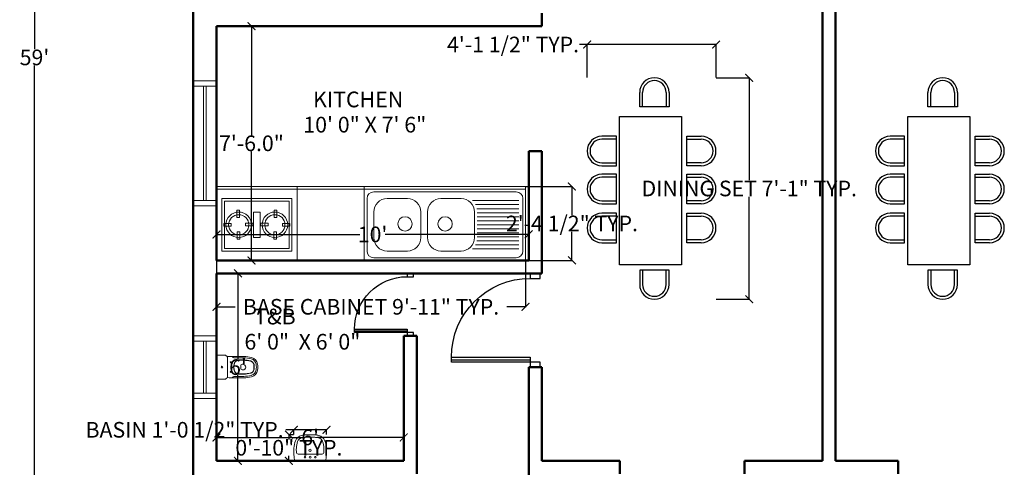
# Model space of a CAD drawing. Units: inches. Extents: x 147 to 1638, y 107 to 941.
# Tile 8 of 17: x 158 to 537, y 398 to 570. Entities that reach past the tile are written whole.
import ezdxf

# ---------------------------------------------------------------- set-up
doc = ezdxf.new("R2010")
doc.units = ezdxf.units.IN
doc.header["$MEASUREMENT"] = 0
for name, color, linetype, lineweight in [('A-ANNO-DIMS', 2, 'Continuous', 15), ('A-AREA-IDEN', 7, 'Continuous', 18), ('A-Door', 150, 'Continuous', 25), ('A-EQPM', 8, 'Continuous', 18), ('A-FLOR-CASE', 9, 'Continuous', 20), ('A-FLOR-FIXT', 9, 'Continuous', 18), ('furniture', 50, 'Continuous', 18), ('walls', 7, 'Continuous', 50), ('windows', 3, 'Continuous', 20)]:
    doc.layers.add(name, color=color, linetype=linetype, lineweight=lineweight)
for name, color, linetype in [('A-Glaz', 92, 'Continuous'), ('NT', 1, 'Continuous'), ('家', 40, 'Continuous')]:
    doc.layers.add(name, color=color, linetype=linetype)
doc.styles.get("Standard").update_dxf_attribs({"font": 'arial.ttf'})
doc.dimstyles.get("Standard").update_dxf_attribs({"dimtxt": 6, "dimasz": 3, "dimexe": 0.18, "dimexo": 0.0625, "dimgap": 0.09, "dimtad": 0, "dimtih": 1, "dimtoh": 1, "dimdec": 1, "dimzin": 0, "dimdsep": 46, "dimlunit": 3, "dimtxsty": 'Standard', "dimblk": 'ARCHTICK', "dimcen": 0.09, "dimadec": 0, "dimazin": 0, "dimtfac": 1, "dimtdec": 1, "dimtofl": 0, "dimtmove": 0, "dimatfit": 3, "dimfxl": 1, "dimtolj": 1, "dimtzin": 0, "dimarcsym": 0})

# ---------------------------------------------------------------- blocks, each defined once
blk = doc.blocks.new('A$C087A3AA9')
at = {"layer": 'A-Door'}
for points in [[(852.6, 94.7), (852.6, 852.6), (805.3, 852.6), (805.3, 94.7)], [(47.4, 94.7), (47.4, 0), (0, 0), (0, 94.7)], [(900, 94.7), (900, 0), (852.6, 0), (852.6, 94.7)]]:
    blk.add_lwpolyline(points, close=True, dxfattribs=at)
at = {"layer": 'A-Glaz'}
blk.add_line((828.9, 852.6), (828.9, 94.7), dxfattribs=at)
at = {"layer": 'NT'}
blk.add_arc((805.3, 94.7), 757.9, 90, 180, dxfattribs=at)
blk = doc.blocks.new('_ArchTick')
at = {"color": 0, "linetype": 'ByBlock', "const_width": 0.15}
blk.add_lwpolyline([(-0.5, -0.5), (0.5, 0.5)], dxfattribs=at)
blk = doc.blocks.new('*D14')
at = {"layer": 'A-ANNO-DIMS', "color": 0, "lineweight": -2, "transparency": 16777216}
for p, q in [((244.71, 567.72), (247.56, 567.72)), ((247.38, 567.72), (247.38, 525.87)), ((247.38, 477.72), (247.38, 519.56)), ((244.71, 477.72), (247.56, 477.72))]:
    blk.add_line(p, q, dxfattribs=at)
at = {"layer": 'Defpoints', "color": 0, "lineweight": -2, "transparency": 16777216}
for p in [(244.65, 567.72), (244.65, 477.72), (247.38, 477.72)]:
    blk.add_point(p, dxfattribs=at)
at = {"layer": 'A-ANNO-DIMS', "color": 0, "lineweight": -2, "transparency": 16777216, "xscale": 3, "yscale": 3, "zscale": 3}
for p, rotation in [((247.38, 567.72), 90), ((247.38, 477.72), 270)]:
    blk.add_blockref('_ArchTick', p, dxfattribs=dict(at, rotation=rotation))
at = {"layer": 'A-ANNO-DIMS', "color": 0, "transparency": 16777216, "insert": (247.38, 522.72), "char_height": 6, "attachment_point": 5}
blk.add_mtext('\\A1;7\'-6.0"', dxfattribs=at)
blk = doc.blocks.new('*D15')
at = {"layer": 'A-ANNO-DIMS', "color": 0, "lineweight": -2, "transparency": 16777216}
for p, q in [((233.94, 487.78), (233.94, 487.9)), ((233.94, 487.72), (289.05, 487.72)), ((353.94, 487.72), (298.84, 487.72)), ((353.94, 487.78), (353.94, 487.9))]:
    blk.add_line(p, q, dxfattribs=at)
at = {"layer": 'Defpoints', "color": 0, "lineweight": -2, "transparency": 16777216}
for p in [(233.94, 487.72), (353.94, 487.72), (353.94, 487.72)]:
    blk.add_point(p, dxfattribs=at)
at = {"layer": 'A-ANNO-DIMS', "color": 0, "lineweight": -2, "transparency": 16777216, "xscale": 3, "yscale": 3, "zscale": 3, "rotation": 180}
blk.add_blockref('_ArchTick', (233.94, 487.72), dxfattribs=at)
at = {"layer": 'A-ANNO-DIMS', "color": 0, "lineweight": -2, "transparency": 16777216, "xscale": 3, "yscale": 3, "zscale": 3}
blk.add_blockref('_ArchTick', (353.94, 487.72), dxfattribs=at)
at = {"layer": 'A-ANNO-DIMS', "color": 0, "transparency": 16777216, "insert": (293.94, 487.72), "char_height": 6, "attachment_point": 5}
blk.add_mtext("\\A1;10'", dxfattribs=at)
blk = doc.blocks.new('*D16')
at = {"layer": 'A-ANNO-DIMS', "color": 0, "lineweight": -2, "transparency": 16777216}
for p, q in [((239.65, 472.72), (242.37, 472.72)), ((242.19, 472.72), (242.19, 439.87)), ((242.19, 400.72), (242.19, 433.56)), ((239.65, 400.72), (242.37, 400.72))]:
    blk.add_line(p, q, dxfattribs=at)
at = {"layer": 'Defpoints', "color": 0, "lineweight": -2, "transparency": 16777216}
for p in [(239.59, 472.72), (239.59, 400.72), (242.19, 400.72)]:
    blk.add_point(p, dxfattribs=at)
at = {"layer": 'A-ANNO-DIMS', "color": 0, "lineweight": -2, "transparency": 16777216, "xscale": 3, "yscale": 3, "zscale": 3}
for p, rotation in [((242.19, 472.72), 90), ((242.19, 400.72), 270)]:
    blk.add_blockref('_ArchTick', p, dxfattribs=dict(at, rotation=rotation))
at = {"layer": 'A-ANNO-DIMS', "color": 0, "transparency": 16777216, "insert": (242.19, 436.72), "char_height": 6, "attachment_point": 5}
blk.add_mtext("\\A1;6'", dxfattribs=at)
blk = doc.blocks.new('*D17')
at = {"layer": 'A-ANNO-DIMS', "color": 0, "lineweight": -2, "transparency": 16777216}
for p, q in [((233.94, 407.58), (233.94, 409.9)), ((233.94, 409.72), (267.08, 409.72)), ((305.94, 409.72), (272.81, 409.72)), ((305.94, 407.58), (305.94, 409.9))]:
    blk.add_line(p, q, dxfattribs=at)
at = {"layer": 'Defpoints', "color": 0, "lineweight": -2, "transparency": 16777216}
for p in [(305.94, 409.72), (233.94, 407.52), (305.94, 407.52)]:
    blk.add_point(p, dxfattribs=at)
at = {"layer": 'A-ANNO-DIMS', "color": 0, "lineweight": -2, "transparency": 16777216, "xscale": 3, "yscale": 3, "zscale": 3, "rotation": 180}
blk.add_blockref('_ArchTick', (233.94, 409.72), dxfattribs=at)
at = {"layer": 'A-ANNO-DIMS', "color": 0, "lineweight": -2, "transparency": 16777216, "xscale": 3, "yscale": 3, "zscale": 3}
blk.add_blockref('_ArchTick', (305.94, 409.72), dxfattribs=at)
at = {"layer": 'A-ANNO-DIMS', "color": 0, "transparency": 16777216, "insert": (269.94, 409.72), "char_height": 6, "attachment_point": 5}
blk.add_mtext("\\A1;6'", dxfattribs=at)
blk = doc.blocks.new('*D70')
at = {"layer": 'A-ANNO-DIMS', "color": 0, "lineweight": -2, "transparency": 16777216}
for p, q in [((224.88, 909.72), (163.8, 909.72)), ((163.98, 909.72), (163.98, 558.87)), ((163.98, 201.72), (163.98, 552.56)), ((224.88, 201.72), (163.8, 201.72))]:
    blk.add_line(p, q, dxfattribs=at)
at = {"layer": 'Defpoints', "color": 0, "lineweight": -2, "transparency": 16777216}
for p in [(224.94, 909.72), (163.98, 201.72), (224.94, 201.72)]:
    blk.add_point(p, dxfattribs=at)
at = {"layer": 'A-ANNO-DIMS', "color": 0, "lineweight": -2, "transparency": 16777216, "xscale": 3, "yscale": 3, "zscale": 3}
for p, rotation in [((163.98, 909.72), 90), ((163.98, 201.72), 270)]:
    blk.add_blockref('_ArchTick', p, dxfattribs=dict(at, rotation=rotation))
at = {"layer": 'A-ANNO-DIMS', "color": 0, "transparency": 16777216, "insert": (163.98, 555.72), "char_height": 6, "attachment_point": 5}
blk.add_mtext("\\A1;59'", dxfattribs=at)
blk = doc.blocks.new('2SAINDA')
at = {"color": 0, "linetype": 'ByBlock'}
for p, q in [((0, 0.188), (0, -0.188)), ((0.018, 0.2), (0.141, 0.2)), ((0.157, 0.192), (0.162, 0.188)), ((0.18, -0.164), (0.18, 0.164)), ((0.279, 0.159), (0.261, 0.176)), ((0.437, 0.047), (0.424, 0.047)), ((0.279, -0.159), (0.261, -0.176)), ((0.437, -0.047), (0.424, -0.047)), ((0.018, -0.2), (0.141, -0.2)), ((0.157, -0.192), (0.162, -0.188))]:
    blk.add_line(p, q, dxfattribs=at)
for centre, radius in [((0.09, 0), 0.0135), ((0.09, 0), 0.0135), ((0.236, 0.08), 0.0075), ((0.236, -0.08), 0.0075)]:
    blk.add_circle(centre, radius, dxfattribs=at)
for centre, radius, start, end in [((0.018, 0.18), 0.02, 90, 155.6901), ((0.141, 0.181), 0.019, 34.9372, 90), ((0.155, 0.164), 0.025, 23.3776, 73.7848), ((0.383, -5.322), 5.5, 89.2905, 92.1362), ((0.155, 0.164), 0.025, 360, 23.3776), ((0.444, -0.373), 0.55, 75.4605, 89.2905), ((0.293, 0.173), 0.02, 225, 270.9364), ((0.485, 0), 0.2, 160.016, 199.984), ((0.485, 0), 0.196, 160.016, 199.984), ((0.383, -5.322), 5.476, 89.2905, 90.9364), ((0.368, 0.043), 0.075, 90.1648, 160.016), ((0.368, 0.043), 0.071, 90.1648, 160.016), ((0.383, -5.322), 5.44, 89.2905, 90.1648), ((0.383, -5.322), 5.436, 89.2905, 90.1648), ((0.582, 0), 0.18, 170.2849, 189.7151), ((0.424, 0.027), 0.02, 90, 170.2849), ((0.437, 0), 0.047, 0, 90), ((0.437, 0), 0.047, 270, 0), ((0.444, -0.373), 0.49, 75.4605, 89.2905), ((0.444, -0.373), 0.486, 75.4605, 89.2905), ((0.444, -0.373), 0.526, 75.4605, 89.2905), ((0.549, 0.03), 0.07, 8.8162, 75.4605), ((0.549, 0.03), 0.074, 8.8162, 75.4605), ((0.549, 0.03), 0.11, 8.8162, 75.4605), ((0.549, 0.03), 0.134, 8.8162, 75.4605), ((0.355, 0), 0.266, 351.1838, 8.8162), ((0.355, 0), 0.27, 351.1838, 8.8162), ((0.355, 0), 0.306, 351.1838, 8.8162), ((0.355, 0), 0.33, 351.1838, 8.8162), ((0.293, -0.173), 0.02, 89.0636, 135), ((0.383, 5.322), 5.476, 269.0636, 270.7095), ((0.368, -0.043), 0.075, 199.984, 269.8352), ((0.368, -0.043), 0.071, 199.984, 269.8352), ((0.383, 5.322), 5.436, 269.8352, 270.7095), ((0.383, 5.322), 5.44, 269.8352, 270.7095), ((0.424, -0.027), 0.02, 189.7151, 270), ((0.444, 0.373), 0.486, 270.7095, 284.5395), ((0.444, 0.373), 0.49, 270.7095, 284.5395), ((0.444, 0.373), 0.526, 270.7095, 284.5395), ((0.444, 0.373), 0.55, 270.7095, 284.5395), ((0.549, -0.03), 0.07, 284.5395, 351.1838), ((0.549, -0.03), 0.074, 284.5395, 351.1838), ((0.549, -0.03), 0.11, 284.5395, 351.1838), ((0.549, -0.03), 0.134, 284.5395, 351.1838), ((0.018, -0.18), 0.02, 204.3099, 270), ((0.141, -0.181), 0.019, 270, 325.0628), ((0.155, -0.164), 0.025, 286.2152, 336.6224), ((0.155, -0.164), 0.025, 336.6224, 0), ((0.383, 5.322), 5.5, 267.8638, 270.7095)]:
    blk.add_arc(centre, radius, start, end, dxfattribs=at)
blk = doc.blocks.new('2SALADA2')
at = {"color": 0}
for p, q in [((-0.296, 0), (0.296, 0)), ((0.207, -0.13), (-0.207, -0.13))]:
    blk.add_line(p, q, dxfattribs=at)
for centre, radius in [((-0.1, -0.07), 0.015), ((0, -0.205), 0.023), ((0, -0.07), 0.0175), ((0.1, -0.07), 0.015)]:
    blk.add_circle(centre, radius, dxfattribs=at)
for centre, radius, start, end in [((-0.296, -0.01), 0.01, 90, 173.6262), ((0.296, -0.01), 0.01, 6.3738, 90), ((1.185, -0.175), 1.5, 173.6262, 182.693), ((1.186, -0.221), 1.454, 178.0234, 180.898), ((-0.227, -0.171), 0.04, 95.5937, 179.6995), ((-0.207, -0.38), 0.25, 90, 95.5937), ((0.207, -0.38), 0.25, 84.4063, 90), ((0.227, -0.171), 0.04, 0.3005, 84.4063), ((-1.186, -0.221), 1.454, 359.102, 1.9766), ((-1.185, -0.175), 1.5, 357.307, 6.3738), ((0.186, -0.222), 0.5, 182.693, 199.3406), ((0.186, -0.222), 0.454, 182.693, 199.3406), ((-0.135, -0.335), 0.114, 199.3406, 257.4429), ((0.135, -0.335), 0.114, 282.5571, 340.6594), ((-0.186, -0.222), 0.454, 340.6594, 357.307), ((-0.186, -0.222), 0.5, 340.6594, 357.307), ((-0.135, -0.335), 0.16, 199.3406, 257.4429), ((-0.061, -0.003), 0.5, 257.4429, 266.4982), ((-0.061, -0.003), 0.454, 257.4429, 266.4982), ((0, 0.995), 1.5, 266.4982, 273.5018), ((0, 0.995), 1.454, 266.4982, 273.5018), ((0.061, -0.003), 0.454, 273.5018, 282.5571), ((0.061, -0.003), 0.5, 273.5018, 282.5571), ((0.135, -0.335), 0.16, 282.5571, 340.6594)]:
    blk.add_arc(centre, radius, start, end, dxfattribs=at)
blk = doc.blocks.new('A$C45A766E2')
at = {"layer": '家'}
for p, q in [((0.363, 1.317), (0.363, 1.078)), ((0.412, 1.317), (0.412, 1.078)), ((0.801, 1.078), (0.801, 1.317)), ((0.849, 1.078), (0.849, 1.317)), ((1.006, 1.317), (1.006, 1.078)), ((1.054, 1.317), (1.054, 1.078)), ((1.443, 1.078), (1.443, 1.317)), ((1.492, 1.078), (1.492, 1.317)), ((1.634, 1.317), (1.634, 1.078)), ((1.683, 1.317), (1.683, 1.078)), ((2.072, 1.078), (2.072, 1.317)), ((2.12, 1.078), (2.12, 1.317)), ((0, 1.028), (2.445, 1.028)), ((0, 0), (0, 1.028)), ((0.363, 1.078), (0.849, 1.078)), ((0.363, 1.078), (0.849, 1.078)), ((1.006, 1.078), (1.492, 1.078)), ((1.006, 1.078), (1.492, 1.078)), ((1.634, 1.078), (2.12, 1.078)), ((1.634, 1.078), (2.12, 1.078)), ((2.445, 1.028), (2.445, 0)), ((-0.088, 0.693), (-0.327, 0.693)), ((-0.088, 0.207), (-0.088, 0.693)), ((-0.088, 0.207), (-0.088, 0.693)), ((2.604, 0.693), (2.843, 0.693)), ((2.604, 0.207), (2.604, 0.693)), ((2.604, 0.207), (2.604, 0.693)), ((-0.088, 0.644), (-0.327, 0.644)), ((2.604, 0.644), (2.843, 0.644)), ((-0.327, 0.255), (-0.088, 0.255)), ((-0.327, 0.207), (-0.088, 0.207)), ((2.843, 0.255), (2.604, 0.255)), ((2.843, 0.207), (2.604, 0.207)), ((2.445, 0), (0, 0)), ((0.363, -0.085), (0.849, -0.085)), ((0.363, -0.085), (0.849, -0.085)), ((0.363, -0.324), (0.363, -0.085)), ((0.412, -0.324), (0.412, -0.085)), ((0.801, -0.085), (0.801, -0.324)), ((0.849, -0.085), (0.849, -0.324)), ((1.006, -0.324), (1.006, -0.085)), ((1.006, -0.085), (1.492, -0.085)), ((1.006, -0.085), (1.492, -0.085)), ((1.054, -0.324), (1.054, -0.085)), ((1.443, -0.085), (1.443, -0.324)), ((1.492, -0.085), (1.492, -0.324)), ((1.634, -0.085), (2.12, -0.085)), ((1.634, -0.085), (2.12, -0.085)), ((1.634, -0.324), (1.634, -0.085)), ((1.683, -0.324), (1.683, -0.085)), ((2.072, -0.085), (2.072, -0.324)), ((2.12, -0.085), (2.12, -0.324))]:
    blk.add_line(p, q, dxfattribs=at)
for centre, radius, start, end in [((0.606, 1.317), 0.243, 0, 180), ((0.606, 1.317), 0.195, 0, 180), ((1.249, 1.317), 0.243, 0, 180), ((1.249, 1.317), 0.195, 0, 180), ((1.877, 1.317), 0.243, 0, 180), ((1.877, 1.317), 0.195, 0, 180), ((-0.327, 0.45), 0.243, 90, 270), ((2.843, 0.45), 0.243, 270, 90), ((-0.327, 0.45), 0.195, 90, 270), ((2.843, 0.45), 0.195, 270, 90), ((0.606, -0.324), 0.243, 180, 0), ((0.606, -0.324), 0.195, 180, 0), ((1.249, -0.324), 0.243, 180, 0), ((1.249, -0.324), 0.195, 180, 0), ((1.877, -0.324), 0.243, 180, 0), ((1.877, -0.324), 0.195, 180, 0)]:
    blk.add_arc(centre, radius, start, end, dxfattribs=at)
blk = doc.blocks.new('WIN-48IN')
for p, q in [((9, 48), (0, 48)), ((0, 48), (0, 0)), ((9, 46), (0, 46)), ((4, 2), (4, 46)), ((5, 2), (5, 46)), ((9, 0), (9, 48)), ((0, 2), (9, 2)), ((0, 0), (9, 0))]:
    blk.add_line(p, q)
blk = doc.blocks.new('WIN-24IN')
for p, q in [((9, 24), (0, 24)), ((0, 24), (0, 0)), ((9, 0), (9, 24)), ((9, 22), (0, 22)), ((4, 2), (4, 22)), ((5, 2), (5, 22)), ((0, 2), (9, 2)), ((0, 0), (9, 0))]:
    blk.add_line(p, q)
blk = doc.blocks.new('CABINET-KITCHEN-RUN')
for p, q in [((0, 28.41), (118.8, 28.41)), ((0, 0), (0, 28.41)), ((0, 27.38), (118.8, 27.38)), ((30.99, 0), (30.99, 28.41)), ((56.82, 0), (56.82, 28.41)), ((118.8, 28.41), (118.8, 0)), ((118.8, 0), (0, 0))]:
    blk.add_line(p, q)
blk = doc.blocks.new('COOKTOP-2-BURNER')
for p, q in [((0, 0), (0, 20.15)), ((0, 20.15), (26.86, 20.15)), ((1.03, 1.03), (1.03, 19.11)), ((1.03, 19.11), (25.83, 19.11)), ((25.83, 1.03), (25.83, 19.11)), ((26.86, 0), (26.86, 20.15)), ((5.75, 15.75), (5.75, 12.91)), ((5.75, 15.75), (6.79, 15.75)), ((6.79, 15.75), (6.79, 12.91)), ((21.11, 15.75), (20.07, 15.75)), ((20.07, 15.75), (20.07, 12.91)), ((21.11, 15.75), (21.11, 12.91)), ((5.75, 12.91), (6.79, 12.91)), ((12.14, 14.98), (14.72, 14.98)), ((12.14, 14.98), (12.14, 5.17)), ((14.72, 14.98), (14.72, 5.17)), ((21.11, 12.91), (20.07, 12.91)), ((0.69, 9.55), (0.69, 10.59)), ((0.69, 10.59), (3.53, 10.59)), ((0.69, 9.55), (3.53, 9.55)), ((3.53, 9.55), (3.53, 10.59)), ((11.95, 10.69), (9.11, 10.69)), ((9.11, 10.69), (9.11, 9.66)), ((11.95, 9.66), (9.11, 9.66)), ((11.95, 10.69), (11.95, 9.66)), ((14.91, 10.69), (17.75, 10.69)), ((14.91, 10.69), (14.91, 9.66)), ((14.91, 9.66), (17.75, 9.66)), ((17.75, 10.69), (17.75, 9.66)), ((23.33, 9.55), (23.33, 10.59)), ((26.17, 10.59), (23.33, 10.59)), ((26.17, 9.55), (23.33, 9.55)), ((26.17, 9.55), (26.17, 10.59)), ((5.86, 4.49), (5.86, 7.33)), ((6.89, 7.33), (5.86, 7.33)), ((6.89, 4.49), (5.86, 4.49)), ((6.89, 4.49), (6.89, 7.33)), ((12.14, 5.17), (14.72, 5.17)), ((19.97, 4.49), (19.97, 7.33)), ((19.97, 7.33), (21, 7.33)), ((19.97, 4.49), (21, 4.49)), ((21, 4.49), (21, 7.33)), ((0, 0), (26.86, 0)), ((1.03, 1.03), (25.83, 1.03))]:
    blk.add_line(p, q)
for centre, radius in [((6.48, 10.08), 4.91), ((6.48, 10.08), 3.87), ((20.38, 10.08), 4.91), ((20.38, 10.08), 3.87)]:
    blk.add_circle(centre, radius)
blk = doc.blocks.new('SINK-DOUBLE-DRAINBOARD')
for p, q in [((0, 22.73), (0, 2.58)), ((57.34, 25.31), (2.58, 25.31)), ((15.5, 22.73), (7.75, 22.73)), ((36.16, 22.73), (28.41, 22.73)), ((59.92, 2.58), (59.92, 22.73)), ((40.53, 21.95), (58.37, 21.95)), ((41.67, 20.4), (58.37, 20.4)), ((2.58, 17.56), (2.58, 7.75)), ((20.66, 17.56), (20.66, 7.75)), ((23.24, 17.56), (23.24, 7.75)), ((41.32, 17.56), (41.32, 7.75)), ((42.22, 18.85), (58.37, 18.85)), ((42.36, 17.3), (58.37, 17.3)), ((42.36, 15.75), (58.37, 15.75)), ((42.36, 14.2), (58.37, 14.2)), ((42.36, 12.66), (58.37, 12.66)), ((42.36, 11.11), (58.37, 11.11)), ((42.36, 9.56), (58.37, 9.56)), ((42.36, 8.01), (58.37, 8.01)), ((41.67, 4.91), (58.37, 4.91)), ((42.22, 6.46), (58.37, 6.46)), ((2.58, 0), (57.34, 0)), ((7.75, 2.58), (15.5, 2.58)), ((28.41, 2.58), (36.16, 2.58)), ((40.53, 3.36), (58.37, 3.36))]:
    blk.add_line(p, q)
for centre in [(14.61, 13), (30.02, 13)]:
    blk.add_circle(centre, 2.75)
for centre, radius, start, end in [((2.58, 22.73), 2.58, 90, 180), ((7.75, 17.56), 5.17, 90, 180), ((15.5, 17.56), 5.17, 0, 90), ((28.41, 17.56), 5.17, 90, 180), ((36.16, 17.56), 5.17, 0, 90), ((57.34, 22.73), 2.58, 0, 90), ((7.75, 7.75), 5.17, 180, 270), ((15.5, 7.75), 5.17, 270, 0), ((28.41, 7.75), 5.17, 180, 270), ((36.16, 7.75), 5.17, 270, 0), ((2.58, 2.58), 2.58, 180, 270), ((57.34, 2.58), 2.58, 270, 0)]:
    blk.add_arc(centre, radius, start, end)
blk = doc.blocks.new('*D114')
at = {"layer": 'A-ANNO-DIMS', "color": 0, "lineweight": -2, "transparency": 16777216}
for p, q in [((426.01, 547.91), (438.9, 547.91)), ((438.72, 547.91), (438.72, 508.55)), ((438.72, 462.8), (438.72, 502.17)), ((426.01, 462.8), (438.9, 462.8))]:
    blk.add_line(p, q, dxfattribs=at)
at = {"layer": 'Defpoints', "color": 0, "lineweight": -2, "transparency": 16777216}
for p in [(425.95, 547.91), (438.72, 547.91), (425.95, 462.8)]:
    blk.add_point(p, dxfattribs=at)
at = {"layer": 'A-ANNO-DIMS', "color": 0, "lineweight": -2, "transparency": 16777216, "xscale": 3, "yscale": 3, "zscale": 3}
for p, rotation in [((438.72, 547.91), 90), ((438.72, 462.8), 270)]:
    blk.add_blockref('_ArchTick', p, dxfattribs=dict(at, rotation=rotation))
at = {"layer": 'A-ANNO-DIMS', "color": 0, "transparency": 16777216, "insert": (438.72, 505.36), "char_height": 6, "attachment_point": 5}
blk.add_mtext('\\A1;DINING SET 7\'-1" TYP.', dxfattribs=at)
blk = doc.blocks.new('*D115')
at = {"layer": 'A-ANNO-DIMS', "color": 0, "lineweight": -2, "transparency": 16777216}
for p, q in [((376.42, 560.68), (373.42, 560.68)), ((376.42, 547.98), (376.42, 560.86)), ((425.95, 560.68), (376.42, 560.68)), ((425.95, 547.98), (425.95, 560.86))]:
    blk.add_line(p, q, dxfattribs=at)
at = {"layer": 'Defpoints', "color": 0, "lineweight": -2, "transparency": 16777216}
for p in [(376.42, 560.68), (376.42, 547.91), (425.95, 547.91)]:
    blk.add_point(p, dxfattribs=at)
at = {"layer": 'A-ANNO-DIMS', "color": 0, "lineweight": -2, "transparency": 16777216, "xscale": 3, "yscale": 3, "zscale": 3, "rotation": 180}
blk.add_blockref('_ArchTick', (376.42, 560.68), dxfattribs=at)
at = {"layer": 'A-ANNO-DIMS', "color": 0, "lineweight": -2, "transparency": 16777216, "xscale": 3, "yscale": 3, "zscale": 3}
blk.add_blockref('_ArchTick', (425.95, 560.68), dxfattribs=at)
at = {"layer": 'A-ANNO-DIMS', "color": 0, "transparency": 16777216, "insert": (347.93, 560.68), "char_height": 6, "attachment_point": 5}
blk.add_mtext('\\A1;4\'-1 1/2" TYP.', dxfattribs=at)
blk = doc.blocks.new('*D120')
at = {"layer": 'A-ANNO-DIMS', "color": 0, "lineweight": -2, "transparency": 16777216}
for p, q in [((263.65, 412.63), (260.65, 412.63)), ((263.65, 410.81), (263.65, 412.81)), ((276.23, 412.63), (263.65, 412.63)), ((276.23, 410.81), (276.23, 412.81))]:
    blk.add_line(p, q, dxfattribs=at)
at = {"layer": 'Defpoints', "color": 0, "lineweight": -2, "transparency": 16777216}
for p in [(263.65, 412.63), (263.65, 410.74), (276.23, 410.74)]:
    blk.add_point(p, dxfattribs=at)
at = {"layer": 'A-ANNO-DIMS', "color": 0, "lineweight": -2, "transparency": 16777216, "xscale": 3, "yscale": 3, "zscale": 3, "rotation": 180}
blk.add_blockref('_ArchTick', (263.65, 412.63), dxfattribs=at)
at = {"layer": 'A-ANNO-DIMS', "color": 0, "lineweight": -2, "transparency": 16777216, "xscale": 3, "yscale": 3, "zscale": 3}
blk.add_blockref('_ArchTick', (276.23, 412.63), dxfattribs=at)
at = {"layer": 'A-ANNO-DIMS', "color": 0, "transparency": 16777216, "insert": (221.68, 412.63), "char_height": 6, "attachment_point": 5}
blk.add_mtext('\\A1;BASIN 1\'-0 1/2" TYP.', dxfattribs=at)
blk = doc.blocks.new('*D121')
at = {"layer": 'A-ANNO-DIMS', "color": 0, "lineweight": -2, "transparency": 16777216}
for p, q in [((263.59, 410.74), (261.59, 410.74)), ((261.77, 410.74), (261.77, 408.88)), ((261.77, 400.72), (261.77, 402.58)), ((263.59, 400.72), (261.59, 400.72))]:
    blk.add_line(p, q, dxfattribs=at)
at = {"layer": 'Defpoints', "color": 0, "lineweight": -2, "transparency": 16777216}
for p in [(263.65, 410.74), (261.77, 400.72), (263.65, 400.72)]:
    blk.add_point(p, dxfattribs=at)
at = {"layer": 'A-ANNO-DIMS', "color": 0, "lineweight": -2, "transparency": 16777216, "xscale": 3, "yscale": 3, "zscale": 3}
for p, rotation in [((261.77, 410.74), 90), ((261.77, 400.72), 270)]:
    blk.add_blockref('_ArchTick', p, dxfattribs=dict(at, rotation=rotation))
at = {"layer": 'A-ANNO-DIMS', "color": 0, "transparency": 16777216, "insert": (261.77, 405.73), "char_height": 6, "attachment_point": 5}
blk.add_mtext('\\A1;0\'-10" TYP.', dxfattribs=at)
blk = doc.blocks.new('*D122')
at = {"layer": 'A-ANNO-DIMS', "color": 0, "lineweight": -2, "transparency": 16777216}
for p, q in [((233.94, 477.66), (233.94, 459.72)), ((352.75, 477.66), (352.75, 459.72)), ((233.94, 459.9), (241.1, 459.9)), ((352.75, 459.9), (345.59, 459.9))]:
    blk.add_line(p, q, dxfattribs=at)
at = {"layer": 'Defpoints', "color": 0, "lineweight": -2, "transparency": 16777216}
for p in [(233.94, 477.72), (352.75, 477.72), (352.75, 459.9)]:
    blk.add_point(p, dxfattribs=at)
at = {"layer": 'A-ANNO-DIMS', "color": 0, "lineweight": -2, "transparency": 16777216, "xscale": 3, "yscale": 3, "zscale": 3, "rotation": 180}
blk.add_blockref('_ArchTick', (233.94, 459.9), dxfattribs=at)
at = {"layer": 'A-ANNO-DIMS', "color": 0, "lineweight": -2, "transparency": 16777216, "xscale": 3, "yscale": 3, "zscale": 3}
blk.add_blockref('_ArchTick', (352.75, 459.9), dxfattribs=at)
at = {"layer": 'A-ANNO-DIMS', "color": 0, "transparency": 16777216, "insert": (293.35, 459.9), "char_height": 6, "attachment_point": 5}
blk.add_mtext('\\A1;BASE CABINET 9\'-11" TYP.', dxfattribs=at)
blk = doc.blocks.new('*D123')
at = {"layer": 'A-ANNO-DIMS', "color": 0, "lineweight": -2, "transparency": 16777216}
for p, q in [((352.81, 506.13), (370.75, 506.13)), ((370.57, 506.13), (370.57, 495.12)), ((370.57, 477.72), (370.57, 488.73)), ((352.81, 477.72), (370.75, 477.72))]:
    blk.add_line(p, q, dxfattribs=at)
at = {"layer": 'Defpoints', "color": 0, "lineweight": -2, "transparency": 16777216}
for p in [(352.75, 506.13), (370.57, 506.13), (352.75, 477.72)]:
    blk.add_point(p, dxfattribs=at)
at = {"layer": 'A-ANNO-DIMS', "color": 0, "lineweight": -2, "transparency": 16777216, "xscale": 3, "yscale": 3, "zscale": 3}
for p, rotation in [((370.57, 506.13), 90), ((370.57, 477.72), 270)]:
    blk.add_blockref('_ArchTick', p, dxfattribs=dict(at, rotation=rotation))
at = {"layer": 'A-ANNO-DIMS', "color": 0, "transparency": 16777216, "insert": (370.57, 491.92), "char_height": 6, "attachment_point": 5}
blk.add_mtext('\\A1;2\'-4 1/2" TYP.', dxfattribs=at)

msp = doc.modelspace()

# ---------------------------------------------------------------- linework, layer by layer
at = {"layer": 'walls'}
for p, q in [((224.94, 909.72), (224.94, 201.72)), ((466.94, 722.72), (466.94, 400.72)), ((471.94, 722.72), (471.94, 400.72)), ((358.94, 572.72), (358.94, 567.72)), ((233.94, 567.72), (353.94, 567.72)), ((233.94, 567.72), (233.94, 477.72)), ((353.94, 567.72), (358.94, 567.72)), ((353.94, 519.72), (353.94, 477.72)), ((353.94, 519.72), (358.94, 519.72)), ((358.94, 519.72), (358.94, 472.72)), ((233.94, 477.72), (353.94, 477.72)), ((233.94, 472.72), (305.94, 472.72)), ((233.94, 472.72), (233.94, 400.72)), ((310.94, 472.72), (305.94, 472.72)), ((310.94, 472.72), (353.94, 472.72)), ((353.94, 472.72), (358.94, 472.72)), ((305.94, 448.72), (305.94, 400.72)), ((310.94, 448.72), (305.94, 448.72)), ((310.94, 448.72), (310.94, 395.72)), ((353.94, 436.72), (353.94, 210.72)), ((353.94, 436.72), (358.94, 436.72)), ((358.94, 436.72), (358.94, 400.72)), ((233.94, 400.72), (305.94, 400.72)), ((358.94, 400.72), (388.94, 400.72)), ((388.94, 400.72), (388.94, 395.72)), ((436.94, 400.72), (436.94, 395.72)), ((436.94, 400.72), (466.94, 400.72)), ((471.94, 400.72), (495.94, 400.72)), ((495.94, 400.72), (495.94, 395.72))]:
    msp.add_line(p, q, dxfattribs=at)

# ---------------------------------------------------------------- block references
at = {"layer": 'A-Door', "rotation": 90}
for p, xscale, yscale, zscale in [((309.71, 472.72), -0.0266666667542921, 0.0266666667542921, 0.0266666667542921), ((358.34, 472.72), -0.0400000000000001, 0.0400000000000001, 0.0400000000000001)]:
    msp.add_blockref('A$C087A3AA9', p, dxfattribs=dict(at, xscale=xscale, yscale=yscale, zscale=zscale))
at = {"layer": 'A-EQPM'}
msp.add_blockref('COOKTOP-2-BURNER', (236.01, 481.33), dxfattribs=at)
at = {"layer": 'A-FLOR-CASE'}
msp.add_blockref('CABINET-KITCHEN-RUN', (233.94, 477.72), dxfattribs=at)
at = {"layer": 'A-FLOR-FIXT'}
msp.add_blockref('SINK-DOUBLE-DRAINBOARD', (291.8, 478.75), dxfattribs=at)
at = {"layer": 'A-FLOR-FIXT', "xscale": 23.19012112898009, "yscale": 23.19012112898009, "zscale": 23.19012112898009}
msp.add_blockref('2SAINDA', (233.94, 436.72), dxfattribs=at)
at = {"layer": 'A-FLOR-FIXT', "xscale": 19.81841434140962, "yscale": 19.81841434140962, "zscale": 19.81841434140962, "rotation": 180}
msp.add_blockref('2SALADA2', (269.94, 400.72), dxfattribs=at)
at = {"layer": 'furniture', "xscale": 23.28367368005433, "yscale": 23.28367368005433, "zscale": 23.28367368005433, "rotation": 90}
for p in [(412.74, 476.07), (523.56, 476.07)]:
    msp.add_blockref('A$C45A766E2', p, dxfattribs=at)
at = {"layer": 'windows'}
for name, p in [('WIN-48IN', (224.94, 498.72)), ('WIN-24IN', (224.94, 424.72))]:
    msp.add_blockref(name, p, dxfattribs=at)

# ---------------------------------------------------------------- texts
at = {"layer": 'A-AREA-IDEN'}
for s, height, p in [('KITCHEN ', 6.031, (271.05, 536.56)), ('  10\' 0" X 7\' 6"', 6.0306, (263.61, 526.87)), ('T&B', 6.031, (248.44, 453.14)), ('  6\' 0"  X 6\' 0"', 6.0306, (240.99, 443.45))]:
    msp.add_text(s, height=height, dxfattribs=at).set_placement(p)

# ---------------------------------------------------------------- dimensions: what is measured, and where the dimension line sits
at = {"layer": 'A-ANNO-DIMS'}
for base, p1, p2, picture, middle in [((163.98, 201.72), (224.94, 909.72), (224.94, 201.72), '*D70', (163.98, 555.72)), ((247.38, 477.72), (244.65, 567.72), (244.65, 477.72), '*D14', (247.38, 522.72)), ((242.19, 400.72), (239.59, 472.72), (239.59, 400.72), '*D16', (242.19, 436.72))]:
    dim = msp.add_linear_dim(base=base, p1=p1, p2=p2, angle=90, dimstyle='Standard', override={"dimclrd": 0, "dimclre": 0, "dimclrt": 0}, dxfattribs=at)
    dim.commit()
    dim.dimension.update_dxf_attribs({"geometry": picture, "text_midpoint": middle})
for base, p1, p2, angle, text, picture, middle in [((376.42, 560.68), (425.95, 547.91), (376.42, 547.91), 180, '<> TYP.', '*D115', (347.93, 560.68)), ((438.72, 547.91), (425.95, 462.8), (425.95, 547.91), 90, 'DINING SET <> TYP.', '*D114', (438.72, 505.36)), ((370.57, 506.13), (352.75, 477.72), (352.75, 506.13), 90, '<> TYP.', '*D123', (370.57, 491.92)), ((263.65, 412.63), (276.23, 410.74), (263.65, 410.74), 180, 'BASIN <> TYP.', '*D120', (221.68, 412.63)), ((261.77, 400.72), (263.65, 410.74), (263.65, 400.72), 270, '<> TYP.', '*D121', (261.77, 405.73))]:
    dim = msp.add_linear_dim(base=base, p1=p1, p2=p2, angle=angle, text=text, dimstyle='Standard', override={"dimdec": 1, "dimlfac": 1, "dimrnd": 0, "dimzin": 1, "dimdsep": 46, "dimlunit": 4, "dimfrac": 2}, dxfattribs=at)
    dim.commit()
    dim.dimension.update_dxf_attribs({"geometry": picture, "text_midpoint": middle})
for base, p1, p2, picture, middle in [((353.94, 487.72), (233.94, 487.72), (353.94, 487.72), '*D15', (293.94, 487.72)), ((305.94, 409.72), (233.94, 407.52), (305.94, 407.52), '*D17', (269.94, 409.72))]:
    dim = msp.add_linear_dim(base=base, p1=p1, p2=p2, dimstyle='Standard', override={"dimclrd": 0, "dimclre": 0, "dimclrt": 0}, dxfattribs=at)
    dim.commit()
    dim.dimension.update_dxf_attribs({"geometry": picture, "text_midpoint": middle})
dim = msp.add_linear_dim(base=(352.75, 459.9), p1=(233.94, 477.72), p2=(352.75, 477.72), text='BASE CABINET <> TYP.', dimstyle='Standard', override={"dimdec": 1, "dimlfac": 1, "dimrnd": 0, "dimzin": 1, "dimdsep": 46, "dimlunit": 4, "dimfrac": 2}, dxfattribs=at)
dim.commit()
dim.dimension.update_dxf_attribs({"geometry": '*D122', "text_midpoint": (293.35, 459.9)})

doc.saveas('drawing.dxf')
